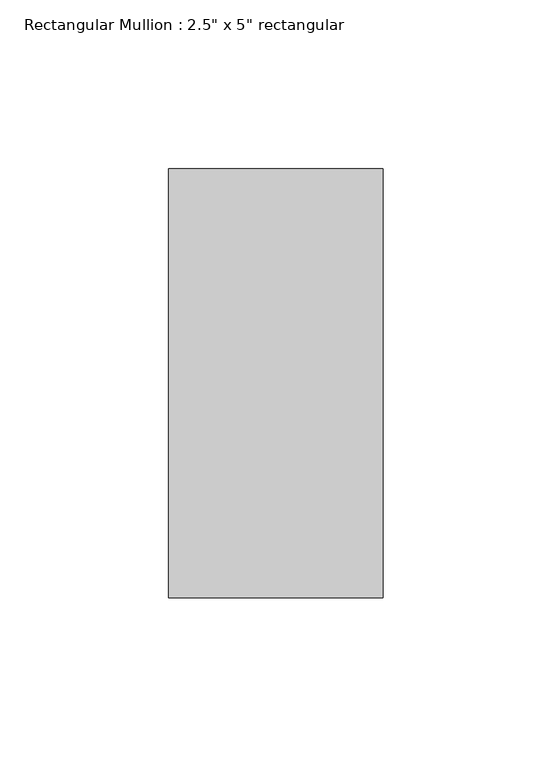
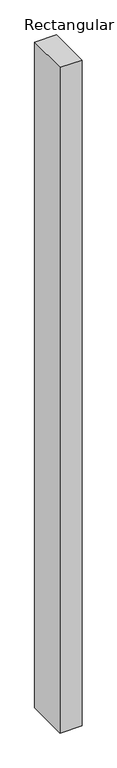
"""IFC4 building model written with IfcOpenShell, lengths in millimetres: member geometry."""

from ifc_helpers import new_model, si_unit, frame, origin, place, context, project, spatial, polyline, outline, extrude, source, transform, mapped, element, save


def member_c8ecc271(model_context):
    return source(origin(), model_context, "Body", "SweptSolid", [
        extrude(outline(polyline([(0.0, 63.5), (0.0, -63.5), (-63.5, -63.5), (-63.5, 63.5), (0.0, 63.5)])), frame((0.0, 0.0, -2038.35), z_axis=(0.0, 0.0, 1.0), x_axis=(1.0, 0.0, 0.0)), (0.0, 0.0, 1.0), 2038.35),
    ])


if __name__ == "__main__":
    model = new_model("IFC4")
    model_context = context("Model", 3, world=origin())
    ifc_project = project(units=[si_unit("LENGTHUNIT", "METRE", prefix="MILLI")], contexts=[model_context])
    site = spatial("IfcSite", under=ifc_project)
    building = spatial("IfcBuilding", under=site)
    placement = place(None, origin())
    member_shape = member_c8ecc271(model_context)
    element("IfcMember", 1, ObjectType="Rectangular Mullion : 2.5\" x 5\" rectangular", at=placement, inside=building, context=model_context, shape_type="MappedRepresentation", body=[
        mapped(member_shape, transform((0.0, 0.0, 0.0), x_axis=(1.0, 0.0, 0.0), y_axis=(0.0, 1.0, 0.0), z_axis=(0.0, 0.0, 1.0))),
    ])
    save(model, "model.ifc")

# Revit data of these elements
# Type "Rectangular Mullion : 2.5\" x 5\" rectangular"
#   built-in parameter 1007304 = 0.416667 (stored number, unit not read)
#   built-in parameter 1007301 = 0.104167 (stored number, unit not read)
#   built-in parameter 1007300 = 0.104167 (stored number, unit not read)
# Element 1 (IfcMember, "Rectangular Mullion : 2.5\" x 5\" rectangular")
#   Materials on its faces: "Aluminum"
# Materials
#   "Aluminum": class "Metal", colour RGB 247 247 247, transparency 0, Description = "Aluminum 6061", Cost = 0
